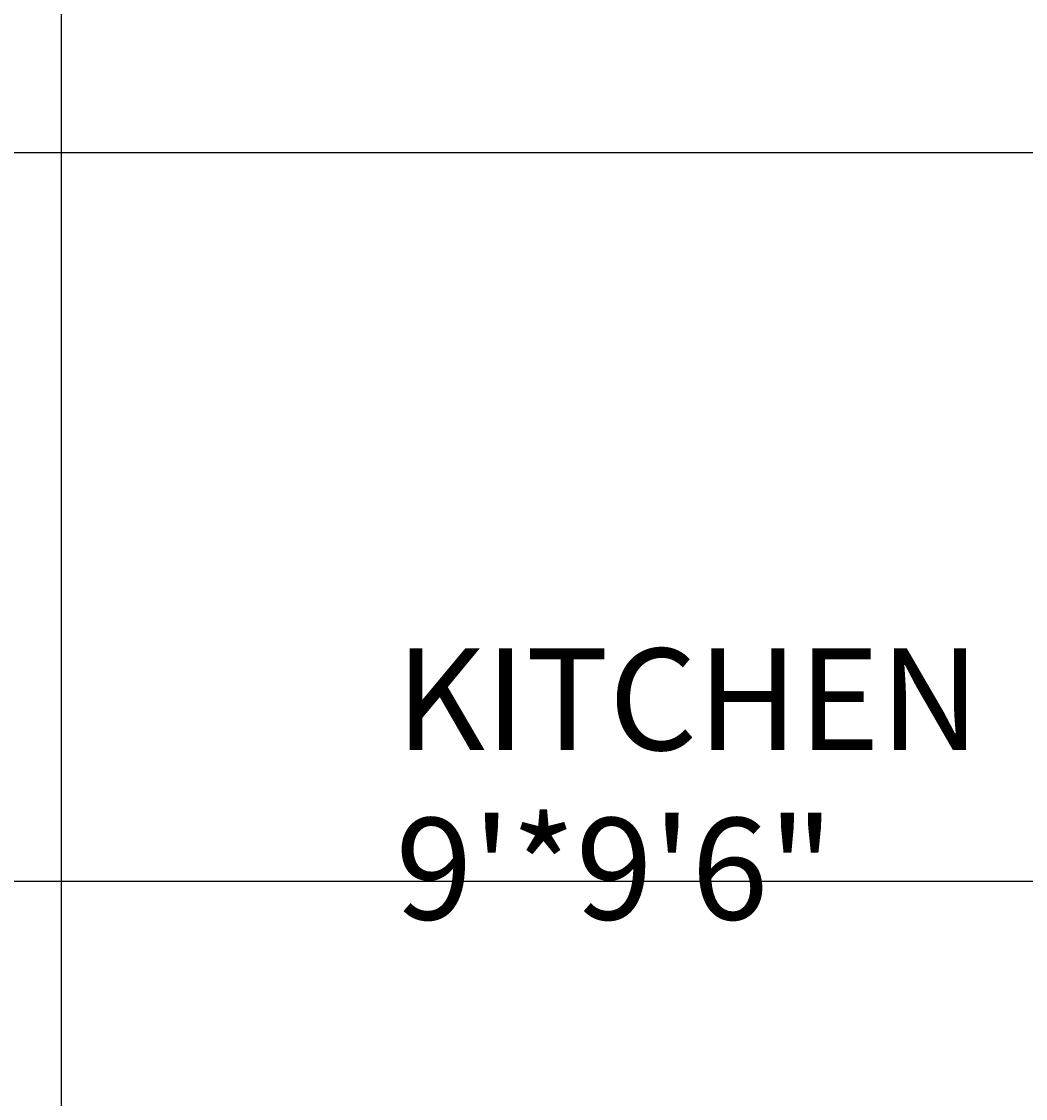
# Model space of a CAD drawing. Units: inches. Extents: x 1998 to 2588, y 1139 to 1977.
# Tile 21 of 134: x 2147 to 2184, y 1629 to 1668. Entities that reach past the tile are written whole.
import ezdxf

# ---------------------------------------------------------------- set-up
doc = ezdxf.new("R2010")
doc.units = ezdxf.units.IN
doc.layers.add('A-ANNO-DIMS', color=2, linetype='Continuous', lineweight=18)
doc.layers.add('A-AREA-IDEN', color=7, linetype='Continuous', lineweight=18)
doc.styles.get("Standard").update_dxf_attribs({"font": 'arial.ttf'})
doc.dimstyles.get("Standard").update_dxf_attribs({"dimtxt": 0.18, "dimasz": 0.18, "dimexe": 0.18, "dimexo": 0.0625, "dimgap": 0.09, "dimtad": 0, "dimtih": 1, "dimtoh": 1, "dimdec": 4, "dimzin": 0, "dimdsep": 46, "dimtxsty": 'Standard', "dimcen": 0.09, "dimadec": 0, "dimazin": 0, "dimtfac": 1, "dimtdec": 4, "dimtofl": 0, "dimtmove": 0, "dimatfit": 3, "dimfxl": 1, "dimtolj": 1, "dimtzin": 0, "dimarcsym": 0})

# ---------------------------------------------------------------- blocks, each defined once
blk = doc.blocks.new('*D30')
at = {"layer": 'A-ANNO-DIMS', "color": 0, "lineweight": -2, "transparency": 16777216}
for p, q in [((2407.91, 1636.732), (1997.843, 1636.732)), ((1998.023, 1636.552), (1998.023, 1615.913)), ((1998.023, 1594.912), (1998.023, 1615.552)), ((2407.91, 1594.732), (1997.843, 1594.732))]:
    blk.add_line(p, q, dxfattribs=at)
at = {"layer": 'A-ANNO-DIMS', "color": 0, "transparency": 16777216}
for points in [[(1997.993, 1636.552), (1998.053, 1636.552), (1998.023, 1636.732)], [(1997.993, 1594.912), (1998.053, 1594.912), (1998.023, 1594.732)]]:
    blk.add_solid(points, dxfattribs=at)
at = {"layer": 'Defpoints', "color": 0, "transparency": 16777216}
for p in [(1998.023, 1636.732), (2407.973, 1636.732), (2407.973, 1594.732)]:
    blk.add_point(p, dxfattribs=at)
at = {"layer": 'A-ANNO-DIMS', "color": 0, "transparency": 16777216, "insert": (1998.023, 1615.732), "char_height": 0.18, "attachment_point": 5}
blk.add_mtext('\\A1;42', dxfattribs=at)
blk = doc.blocks.new('*D37')
at = {"layer": 'A-ANNO-DIMS', "color": 0, "lineweight": -2, "transparency": 16777216}
for p, q in [((2148.455, 1612.795), (2148.455, 1977.362)), ((2197.45, 1612.795), (2197.45, 1977.362)), ((2148.635, 1977.182), (2172.73, 1977.182)), ((2197.27, 1977.182), (2173.175, 1977.182))]:
    blk.add_line(p, q, dxfattribs=at)
at = {"layer": 'A-ANNO-DIMS', "color": 0, "transparency": 16777216}
for points in [[(2148.635, 1977.212), (2148.635, 1977.152), (2148.455, 1977.182)], [(2197.27, 1977.212), (2197.27, 1977.152), (2197.45, 1977.182)]]:
    blk.add_solid(points, dxfattribs=at)
at = {"layer": 'Defpoints', "color": 0, "transparency": 16777216}
for p in [(2197.45, 1977.182), (2148.455, 1612.732), (2197.45, 1612.732)]:
    blk.add_point(p, dxfattribs=at)
at = {"layer": 'A-ANNO-DIMS', "color": 0, "transparency": 16777216, "insert": (2172.952, 1977.182), "char_height": 0.18, "attachment_point": 5}
blk.add_mtext('\\A1;49', dxfattribs=at)
blk = doc.blocks.new('*D38')
at = {"layer": 'A-ANNO-DIMS', "color": 0, "lineweight": -2, "transparency": 16777216}
for p, q in [((2197.387, 1663.247), (1997.843, 1663.247)), ((1998.023, 1663.067), (1998.023, 1638.171)), ((1998.023, 1612.912), (1998.023, 1637.808)), ((2197.387, 1612.732), (1997.843, 1612.732))]:
    blk.add_line(p, q, dxfattribs=at)
at = {"layer": 'A-ANNO-DIMS', "color": 0, "transparency": 16777216}
for points in [[(1997.993, 1663.067), (1998.053, 1663.067), (1998.023, 1663.247)], [(1997.993, 1612.912), (1998.053, 1612.912), (1998.023, 1612.732)]]:
    blk.add_solid(points, dxfattribs=at)
at = {"layer": 'Defpoints', "color": 0, "transparency": 16777216}
for p in [(1998.023, 1663.247), (2197.45, 1663.247), (2197.45, 1612.732)]:
    blk.add_point(p, dxfattribs=at)
at = {"layer": 'A-ANNO-DIMS', "color": 0, "transparency": 16777216, "insert": (1998.023, 1637.99), "char_height": 0.18, "attachment_point": 5}
blk.add_mtext('\\A1;50.51', dxfattribs=at)

msp = doc.modelspace()

# ---------------------------------------------------------------- texts
at = {"layer": 'A-AREA-IDEN', "insert": (2160.6182, 1645.2071), "char_height": 3.69875, "attachment_point": 1}
msp.add_mtext_dynamic_manual_height_columns('KITCHEN\\P9\'*9\'6"', width=110.572713, gutter_width=18.4938, heights=[0], dxfattribs=at)

# ---------------------------------------------------------------- dimensions: what is measured, and where the dimension line sits
at = {"layer": 'A-ANNO-DIMS'}
dim = msp.add_linear_dim(base=(2197.4499, 1977.1824), p1=(2148.4548, 1612.7324), p2=(2197.4499, 1612.7324), dimstyle='Standard', override={"dimdec": 0, "dimlfac": 1, "dimrnd": 0, "dimzin": 0, "dimdsep": 46, "dimlunit": 2}, dxfattribs=at)
dim.commit()
dim.dimension.update_dxf_attribs({"geometry": '*D37', "text_midpoint": (2172.9524, 1977.1824)})
for base, p1, p2, override, picture, middle in [((1998.0229, 1663.2466), (2197.4499, 1612.7324), (2197.4499, 1663.2466), {"dimdec": 2, "dimlfac": 1, "dimrnd": 0, "dimzin": 0, "dimdsep": 46, "dimlunit": 2}, '*D38', (1998.0229, 1637.9895)), ((1998.0229, 1636.7324), (2407.9729, 1594.7324), (2407.9729, 1636.7324), {"dimdec": 0, "dimlfac": 1, "dimrnd": 0, "dimzin": 0, "dimdsep": 46, "dimlunit": 2}, '*D30', (1998.0229, 1615.7324))]:
    dim = msp.add_linear_dim(base=base, p1=p1, p2=p2, angle=90, dimstyle='Standard', override=override, dxfattribs=at)
    dim.commit()
    dim.dimension.update_dxf_attribs({"geometry": picture, "text_midpoint": middle})

doc.saveas('drawing.dxf')
